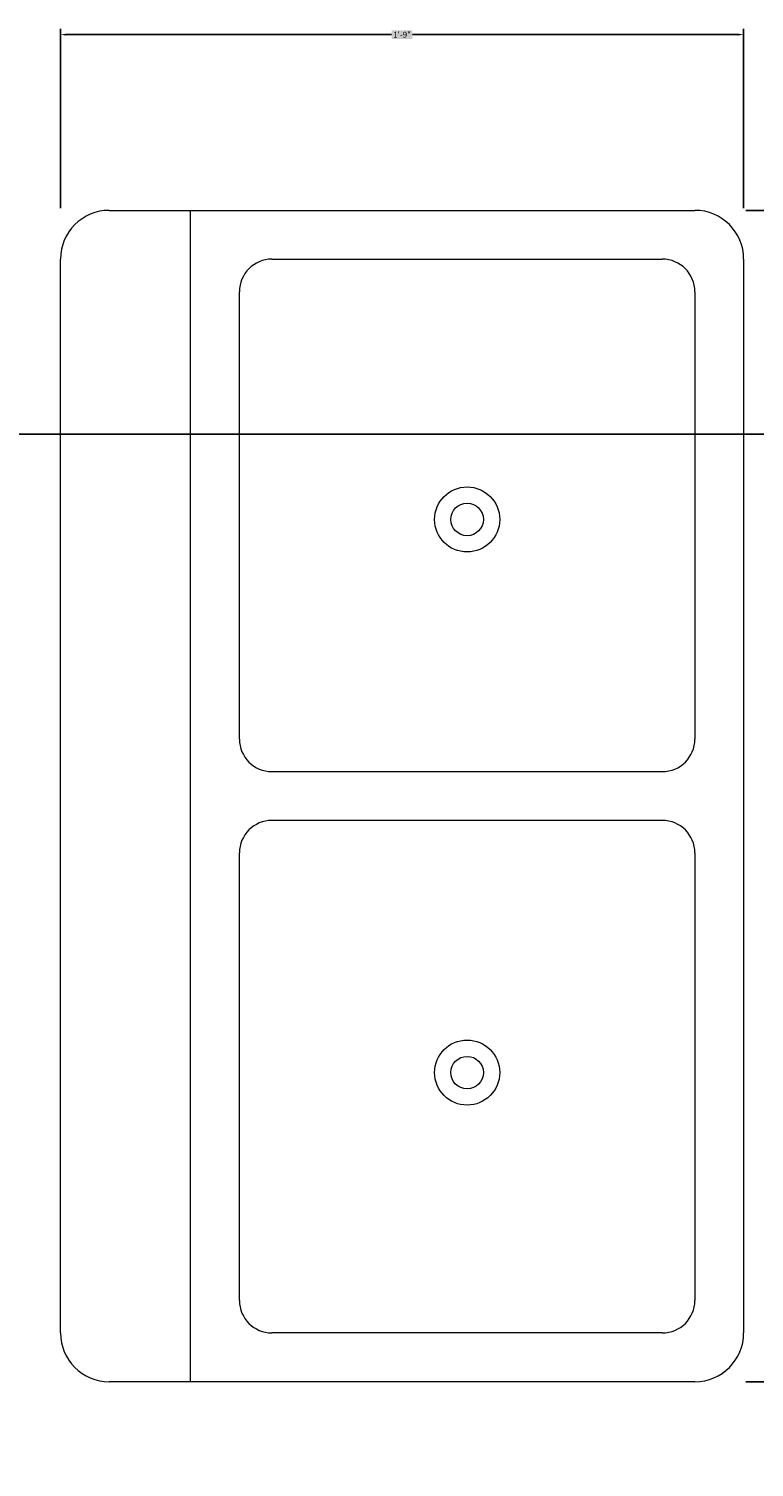
# Model space of a CAD drawing. Units: inches. Extents: x -301 to 715, y -607 to 364.
# Tile 121 of 141: x 101 to 124, y 230 to 274. Entities that reach past the tile are written whole.
import ezdxf

# ---------------------------------------------------------------- set-up
doc = ezdxf.new("R2010")
doc.units = ezdxf.units.IN
doc.header["$MEASUREMENT"] = 0
doc.layers.add('A-ANNO-DIMS', color=2, linetype='Continuous', lineweight=18)
doc.layers.add('A-FLOR-FIXT', color=9, linetype='Continuous', lineweight=18)
doc.styles.get("Standard").update_dxf_attribs({"font": 'arial.ttf'})
doc.dimstyles.get("Standard").update_dxf_attribs({"dimtxt": 0.18, "dimasz": 0.18, "dimexe": 0.18, "dimexo": 0.0625, "dimgap": 0.09, "dimtad": 0, "dimtih": 1, "dimtoh": 1, "dimdec": 1, "dimzin": 0, "dimdsep": 46, "dimlunit": 4, "dimtxsty": 'Standard', "dimcen": 0.09, "dimclrd": 3, "dimclre": 4, "dimclrt": 6, "dimadec": 0, "dimazin": 0, "dimtfac": 1, "dimtdec": 1, "dimtofl": 0, "dimtmove": 0, "dimatfit": 3, "dimfxl": 1, "dimtfill": 2, "dimtfillclr": 51, "dimtolj": 1, "dimtzin": 0, "dimarcsym": 0})

# ---------------------------------------------------------------- blocks, each defined once
blk = doc.blocks.new('Sink-double - 36 in top')
for p, q in [((-18, -4), (18, -4)), ((-0.75, -18.5), (-0.75, -6.5)), ((0.75, -6.5), (0.75, -18.5))]:
    blk.add_line(p, q)
for points in [[(-16.5, 0), (16.5, 0)], [(-18, -19.5), (-18, -1.5)], [(18, -1.5), (18, -19.5)], [(-15.5, -5.5), (-1.75, -5.5)], [(1.75, -5.5), (15.5, -5.5)], [(-16.5, -18.5), (-16.5, -6.5)], [(16.5, -6.5), (16.5, -18.5)], [(-1.75, -19.5), (-15.5, -19.5)], [(15.5, -19.5), (1.75, -19.5)], [(16.5, -21), (-16.5, -21)]]:
    blk.add_lwpolyline(points)
for centre, radius in [((-8.5, -12.5), 1), ((8.5, -12.5), 1), ((-8.5, -12.5), 0.5), ((8.5, -12.5), 0.5)]:
    blk.add_circle(centre, radius)
for centre, radius, start, end in [((-16.5, -1.5), 1.5, 90, 180), ((16.5, -1.5), 1.5, 0, 90), ((-15.5, -6.5), 1, 90, 180), ((-1.75, -6.5), 1, 0, 90), ((1.75, -6.5), 1, 90, 180), ((15.5, -6.5), 1, 0, 90), ((-15.5, -18.5), 1, 180, 270), ((-1.75, -18.5), 1, 270, 0), ((1.75, -18.5), 1, 180, 270), ((15.5, -18.5), 1, 270, 0), ((-16.5, -19.5), 1.5, 180, 270), ((16.5, -19.5), 1.5, 270, 0)]:
    blk.add_arc(centre, radius, start, end)
blk = doc.blocks.new('*D142')
at = {"layer": 'A-ANNO-DIMS', "color": 4, "lineweight": -2, "transparency": 16777216}
for p, q in [((123.308, 268.311), (128.826, 268.311)), ((123.308, 232.311), (128.826, 232.311))]:
    blk.add_line(p, q, dxfattribs=at)
at = {"layer": 'A-ANNO-DIMS', "color": 3, "lineweight": -2, "transparency": 16777216}
for p, q in [((128.646, 268.131), (128.646, 250.494)), ((128.646, 232.491), (128.646, 250.128))]:
    blk.add_line(p, q, dxfattribs=at)
at = {"layer": 'A-ANNO-DIMS', "color": 3, "transparency": 16777216}
for points in [[(128.616, 268.131), (128.676, 268.131), (128.646, 268.311)], [(128.616, 232.491), (128.676, 232.491), (128.646, 232.311)]]:
    blk.add_solid(points, dxfattribs=at)
at = {"layer": 'Defpoints', "color": 0, "transparency": 16777216}
for p in [(123.246, 268.311), (128.646, 268.311), (123.246, 232.311)]:
    blk.add_point(p, dxfattribs=at)
at = {"layer": 'A-ANNO-DIMS', "color": 6, "transparency": 16777216, "insert": (128.646, 250.311), "char_height": 0.18, "attachment_point": 5, "bg_fill": 1, "box_fill_scale": 1.25, "bg_fill_color": 51, "bg_fill_transparency": 0}
blk.add_mtext('\\A1;KITCHEN SINK 3\'-0"', dxfattribs=at)
blk = doc.blocks.new('*D143')
at = {"layer": 'A-ANNO-DIMS', "color": 4, "lineweight": -2, "transparency": 16777216}
for p, q in [((102.246, 268.374), (102.246, 273.891)), ((123.246, 268.374), (123.246, 273.891))]:
    blk.add_line(p, q, dxfattribs=at)
at = {"layer": 'A-ANNO-DIMS', "color": 3, "lineweight": -2, "transparency": 16777216}
for p, q in [((102.426, 273.711), (112.425, 273.711)), ((123.066, 273.711), (113.066, 273.711))]:
    blk.add_line(p, q, dxfattribs=at)
at = {"layer": 'A-ANNO-DIMS', "color": 3, "transparency": 16777216}
for points in [[(102.426, 273.741), (102.426, 273.681), (102.246, 273.711)], [(123.066, 273.741), (123.066, 273.681), (123.246, 273.711)]]:
    blk.add_solid(points, dxfattribs=at)
at = {"layer": 'Defpoints', "color": 0, "transparency": 16777216}
for p in [(102.246, 273.711), (102.246, 268.311), (123.246, 268.311)]:
    blk.add_point(p, dxfattribs=at)
at = {"layer": 'A-ANNO-DIMS', "color": 6, "transparency": 16777216, "insert": (112.746, 273.711), "char_height": 0.18, "attachment_point": 5, "bg_fill": 1, "box_fill_scale": 1.25, "bg_fill_color": 51, "bg_fill_transparency": 0}
blk.add_mtext('\\A1;1\'-9"', dxfattribs=at)
blk = doc.blocks.new('*D157')
at = {"layer": 'A-ANNO-DIMS', "color": 4, "lineweight": -2, "transparency": 16777216}
for p, q in [((-50.541, 261.432), (233.659, 261.432)), ((-50.541, 221.682), (233.659, 221.682))]:
    blk.add_line(p, q, dxfattribs=at)
at = {"layer": 'A-ANNO-DIMS', "color": 3, "lineweight": -2, "transparency": 16777216}
for p, q in [((233.479, 261.252), (233.479, 241.739)), ((233.479, 221.862), (233.479, 241.375))]:
    blk.add_line(p, q, dxfattribs=at)
at = {"layer": 'A-ANNO-DIMS', "color": 3, "transparency": 16777216}
for points in [[(233.449, 261.252), (233.509, 261.252), (233.479, 261.432)], [(233.449, 221.862), (233.509, 221.862), (233.479, 221.682)]]:
    blk.add_solid(points, dxfattribs=at)
at = {"layer": 'Defpoints', "color": 0, "transparency": 16777216}
for p in [(-50.603, 261.432), (233.479, 261.432), (-50.603, 221.682)]:
    blk.add_point(p, dxfattribs=at)
at = {"layer": 'A-ANNO-DIMS', "color": 6, "transparency": 16777216, "insert": (233.479, 241.557), "char_height": 0.18, "attachment_point": 5, "bg_fill": 1, "box_fill_scale": 1.25, "bg_fill_color": 51, "bg_fill_transparency": 0}
blk.add_mtext('\\A1;3\'-4"', dxfattribs=at)

msp = doc.modelspace()

# ---------------------------------------------------------------- block references
at = {"layer": 'A-FLOR-FIXT', "rotation": 90}
msp.add_blockref('Sink-double - 36 in top', (102.246, 250.311), dxfattribs=at)

# ---------------------------------------------------------------- dimensions: what is measured, and where the dimension line sits
at = {"layer": 'A-ANNO-DIMS'}
for base, p1, p2, angle, picture, middle in [((102.246, 273.711), (123.246, 268.311), (102.246, 268.311), 180, '*D143', (112.746, 273.711)), ((233.479242, 261.43233), (-50.603288, 221.68233), (-50.603288, 261.43233), 90, '*D157', (233.479242, 241.55733))]:
    dim = msp.add_linear_dim(base=base, p1=p1, p2=p2, angle=angle, dimstyle='Standard', override={"dimdec": 1, "dimlfac": 1, "dimrnd": 0, "dimzin": 1, "dimdsep": 46, "dimlunit": 4, "dimfrac": 2}, dxfattribs=at)
    dim.commit()
    dim.dimension.update_dxf_attribs({"geometry": picture, "text_midpoint": middle})
dim = msp.add_linear_dim(base=(128.646, 268.311), p1=(123.246, 232.311), p2=(123.246, 268.311), angle=90, text='KITCHEN SINK <>', dimstyle='Standard', override={"dimdec": 1, "dimlfac": 1, "dimrnd": 0, "dimzin": 1, "dimdsep": 46, "dimlunit": 4, "dimfrac": 2}, dxfattribs=at)
dim.commit()
dim.dimension.update_dxf_attribs({"geometry": '*D142', "text_midpoint": (128.646, 250.311)})

doc.saveas('drawing.dxf')
